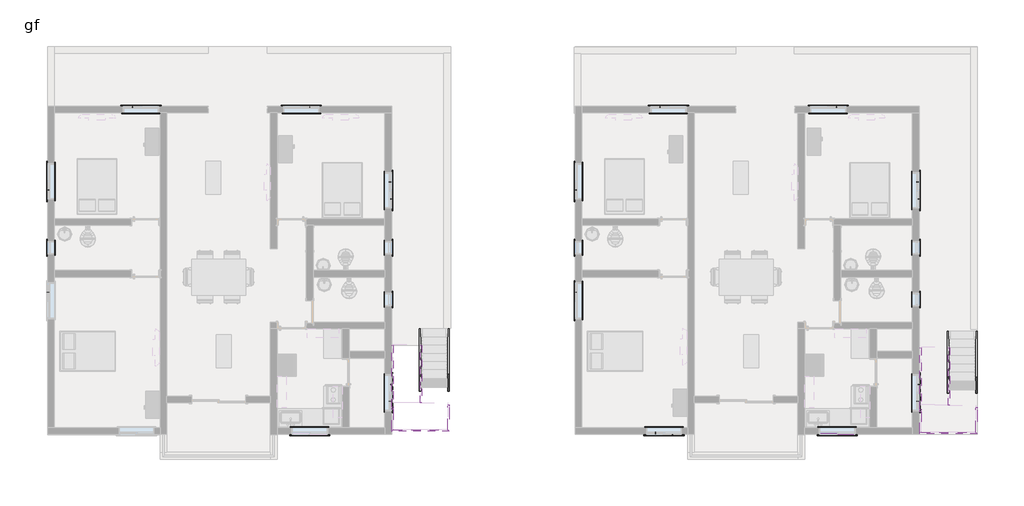
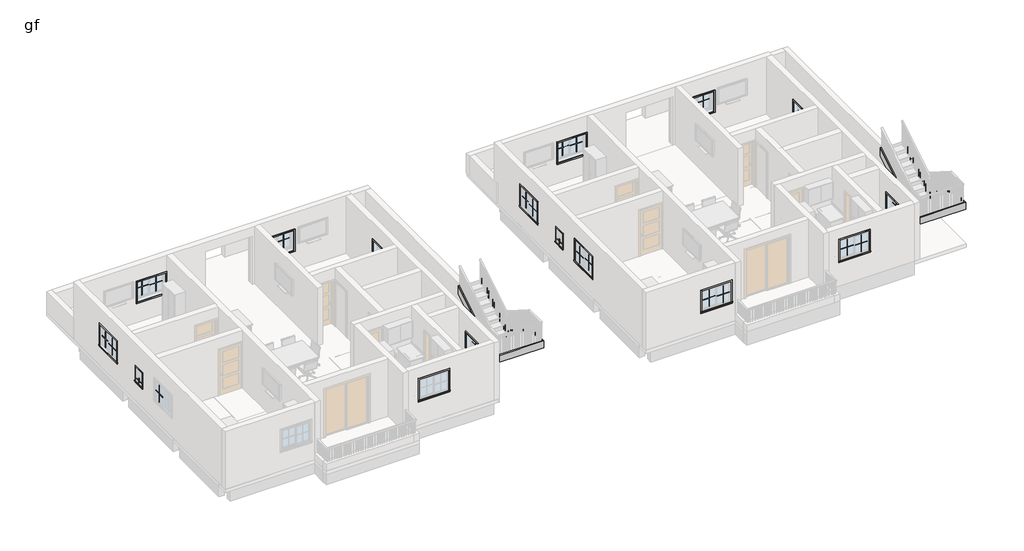
# One storey, part 8 of 8: 73 proxies, 14 members.
"""IFC4 building model written with IfcOpenShell, lengths in millimetres."""

from ifc_helpers import new_model, si_unit, frame, origin, place, context, project, spatial, polyline, outline, extrude, faceted_brep, transform, mapped, element, save
from components import muntin_pattern_2x2_muntin_pattern_2x2_0ac132d2, muntin_pattern_2x2_muntin_pattern_2x2_1fb5fae3, muntin_pattern_2x2_muntin_pattern_2x2_bb7dbb97, trim_window_exterior_flat_with_sill_c4e67c73, trim_window_exterior_flat_with_sill_729ce974, trim_window_exterior_flat_with_sill_e496db69, trim_window_interior_flat_picture_frame_cf1733af, trim_window_interior_flat_picture_frame_5593adf3, trim_window_interior_flat_picture_frame_58837336

model = new_model("IFC4")

# Units and contexts
model_context = context("Model", 3, world=origin())
ifc_project = project(units=[si_unit("LENGTHUNIT", "METRE", prefix="MILLI")], contexts=[model_context])

# Site, building, storey
site = spatial("IfcSite", under=ifc_project)
building = spatial("IfcBuilding", under=site)
storey = spatial("IfcBuildingStorey", under=building, Name="gf", Elevation=609.6)

# Proxies
placement = place(None, origin())
muntin_pattern_2x2_muntin_pattern_2x2_shape = muntin_pattern_2x2_muntin_pattern_2x2_0ac132d2(model_context)
element("IfcBuildingElementProxy", 1, Name="Muntin Pattern_2x2 : Muntin Pattern_2x2", ObjectType="Muntin Pattern_2x2 : Muntin Pattern_2x2", at=placement, inside=storey, context=model_context, shape_type="MappedRepresentation", body=[
    mapped(muntin_pattern_2x2_muntin_pattern_2x2_shape, transform((-12854.1368763, 6465.9185985, 1606.55), x_axis=(1.0, 0.0, 0.0), y_axis=(0.0, 1.0, 0.0), z_axis=(0.0, 0.0, 1.0))),
])
element("IfcBuildingElementProxy", 2, Name="Muntin Pattern_2x2 : Muntin Pattern_2x2", ObjectType="Muntin Pattern_2x2 : Muntin Pattern_2x2", at=placement, inside=storey, context=model_context, shape_type="MappedRepresentation", body=[
    mapped(muntin_pattern_2x2_muntin_pattern_2x2_shape, transform((-13422.4618763, 6510.3685985, 1606.55), x_axis=(1.0, 0.0, 0.0), y_axis=(0.0, 1.0, 0.0), z_axis=(0.0, 0.0, 1.0))),
])
element("IfcBuildingElementProxy", 3, Name="Muntin Pattern_2x2 : Muntin Pattern_2x2", ObjectType="Muntin Pattern_2x2 : Muntin Pattern_2x2", at=placement, inside=storey, context=model_context, shape_type="MappedRepresentation", body=[
    mapped(muntin_pattern_2x2_muntin_pattern_2x2_shape, transform((-16246.6243763, 4251.3560985, 1606.55), x_axis=(0.0, 1.0, 0.0), y_axis=(-1.0, 0.0, 0.0), z_axis=(0.0, 0.0, 1.0))),
])
element("IfcBuildingElementProxy", 4, Name="Muntin Pattern_2x2 : Muntin Pattern_2x2", ObjectType="Muntin Pattern_2x2 : Muntin Pattern_2x2", at=placement, inside=storey, context=model_context, shape_type="MappedRepresentation", body=[
    mapped(muntin_pattern_2x2_muntin_pattern_2x2_shape, transform((-16291.0743763, 3683.0310985, 1606.55), x_axis=(0.0, 1.0, 0.0), y_axis=(-1.0, 0.0, 0.0), z_axis=(0.0, 0.0, 1.0))),
])
element("IfcBuildingElementProxy", 5, Name="Muntin Pattern_2x2 : Muntin Pattern_2x2", ObjectType="Muntin Pattern_2x2 : Muntin Pattern_2x2", at=placement, inside=storey, context=model_context, shape_type="MappedRepresentation", body=[
    mapped(muntin_pattern_2x2_muntin_pattern_2x2_shape, transform((-4695.9743763, -3479.7689015, 1606.55), x_axis=(0.0, -1.0, 0.0), y_axis=(1.0, 0.0, 0.0), z_axis=(0.0, 0.0, 1.0))),
])
element("IfcBuildingElementProxy", 6, Name="Muntin Pattern_2x2 : Muntin Pattern_2x2", ObjectType="Muntin Pattern_2x2 : Muntin Pattern_2x2", at=placement, inside=storey, context=model_context, shape_type="MappedRepresentation", body=[
    mapped(muntin_pattern_2x2_muntin_pattern_2x2_shape, transform((-4651.5243763, -2911.4439015, 1606.55), x_axis=(0.0, -1.0, 0.0), y_axis=(1.0, 0.0, 0.0), z_axis=(0.0, 0.0, 1.0))),
])
element("IfcBuildingElementProxy", 7, Name="Muntin Pattern_2x2 : Muntin Pattern_2x2", ObjectType="Muntin Pattern_2x2 : Muntin Pattern_2x2", at=placement, inside=storey, context=model_context, shape_type="MappedRepresentation", body=[
    mapped(muntin_pattern_2x2_muntin_pattern_2x2_shape, transform((10167.1136273, -4551.3314015, 1835.15), x_axis=(-1.0, 0.0, 0.0), y_axis=(0.0, -1.0, 0.0), z_axis=(0.0, 0.0, 1.0))),
])
element("IfcBuildingElementProxy", 8, Name="Muntin Pattern_2x2 : Muntin Pattern_2x2", ObjectType="Muntin Pattern_2x2 : Muntin Pattern_2x2", at=placement, inside=storey, context=model_context, shape_type="MappedRepresentation", body=[
    mapped(muntin_pattern_2x2_muntin_pattern_2x2_shape, transform((10735.4386273, -4595.7814015, 1835.15), x_axis=(-1.0, 0.0, 0.0), y_axis=(0.0, -1.0, 0.0), z_axis=(0.0, 0.0, 1.0))),
])
element("IfcBuildingElementProxy", 9, Name="Muntin Pattern_2x2 : Muntin Pattern_2x2", ObjectType="Muntin Pattern_2x2 : Muntin Pattern_2x2", at=placement, inside=storey, context=model_context, shape_type="MappedRepresentation", body=[
    mapped(muntin_pattern_2x2_muntin_pattern_2x2_shape, transform((5020.4386273, 6465.9185985, 1606.55), x_axis=(1.0, 0.0, 0.0), y_axis=(0.0, 1.0, 0.0), z_axis=(0.0, 0.0, 1.0))),
])
element("IfcBuildingElementProxy", 10, Name="Muntin Pattern_2x2 : Muntin Pattern_2x2", ObjectType="Muntin Pattern_2x2 : Muntin Pattern_2x2", at=placement, inside=storey, context=model_context, shape_type="MappedRepresentation", body=[
    mapped(muntin_pattern_2x2_muntin_pattern_2x2_shape, transform((4452.1136273, 6510.3685985, 1606.55), x_axis=(1.0, 0.0, 0.0), y_axis=(0.0, 1.0, 0.0), z_axis=(0.0, 0.0, 1.0))),
])
element("IfcBuildingElementProxy", 11, Name="Muntin Pattern_2x2 : Muntin Pattern_2x2", ObjectType="Muntin Pattern_2x2 : Muntin Pattern_2x2", at=placement, inside=storey, context=model_context, shape_type="MappedRepresentation", body=[
    mapped(muntin_pattern_2x2_muntin_pattern_2x2_shape, transform((1627.9511273, 4251.3560985, 1606.55), x_axis=(0.0, 1.0, 0.0), y_axis=(-1.0, 0.0, 0.0), z_axis=(0.0, 0.0, 1.0))),
])
element("IfcBuildingElementProxy", 12, Name="Muntin Pattern_2x2 : Muntin Pattern_2x2", ObjectType="Muntin Pattern_2x2 : Muntin Pattern_2x2", at=placement, inside=storey, context=model_context, shape_type="MappedRepresentation", body=[
    mapped(muntin_pattern_2x2_muntin_pattern_2x2_shape, transform((1583.5011273, 3683.0310985, 1606.55), x_axis=(0.0, 1.0, 0.0), y_axis=(-1.0, 0.0, 0.0), z_axis=(0.0, 0.0, 1.0))),
])
element("IfcBuildingElementProxy", 13, Name="Muntin Pattern_2x2 : Muntin Pattern_2x2", ObjectType="Muntin Pattern_2x2 : Muntin Pattern_2x2", at=placement, inside=storey, context=model_context, shape_type="MappedRepresentation", body=[
    mapped(muntin_pattern_2x2_muntin_pattern_2x2_shape, transform((4299.7136273, -4551.3314015, 1606.55), x_axis=(-1.0, 0.0, 0.0), y_axis=(0.0, -1.0, 0.0), z_axis=(0.0, 0.0, 1.0))),
])
element("IfcBuildingElementProxy", 14, Name="Muntin Pattern_2x2 : Muntin Pattern_2x2", ObjectType="Muntin Pattern_2x2 : Muntin Pattern_2x2", at=placement, inside=storey, context=model_context, shape_type="MappedRepresentation", body=[
    mapped(muntin_pattern_2x2_muntin_pattern_2x2_shape, transform((4868.0386273, -4595.7814015, 1606.55), x_axis=(-1.0, 0.0, 0.0), y_axis=(0.0, -1.0, 0.0), z_axis=(0.0, 0.0, 1.0))),
])
element("IfcBuildingElementProxy", 15, Name="Muntin Pattern_2x2 : Muntin Pattern_2x2", ObjectType="Muntin Pattern_2x2 : Muntin Pattern_2x2", at=placement, inside=storey, context=model_context, shape_type="MappedRepresentation", body=[
    mapped(muntin_pattern_2x2_muntin_pattern_2x2_shape, transform((13178.6011273, -3479.7689015, 1606.55), x_axis=(0.0, -1.0, 0.0), y_axis=(1.0, 0.0, 0.0), z_axis=(0.0, 0.0, 1.0))),
])
element("IfcBuildingElementProxy", 16, Name="Muntin Pattern_2x2 : Muntin Pattern_2x2", ObjectType="Muntin Pattern_2x2 : Muntin Pattern_2x2", at=placement, inside=storey, context=model_context, shape_type="MappedRepresentation", body=[
    mapped(muntin_pattern_2x2_muntin_pattern_2x2_shape, transform((13223.0511273, -2911.4439015, 1606.55), x_axis=(0.0, -1.0, 0.0), y_axis=(1.0, 0.0, 0.0), z_axis=(0.0, 0.0, 1.0))),
])
muntin_pattern_2x2_muntin_pattern_2x2_2_shape = muntin_pattern_2x2_muntin_pattern_2x2_1fb5fae3(model_context)
element("IfcBuildingElementProxy", 17, Name="Muntin Pattern_2x2 : Muntin Pattern_2x2", ObjectType="Muntin Pattern_2x2 : Muntin Pattern_2x2", at=placement, inside=storey, context=model_context, shape_type="MappedRepresentation", body=[
    mapped(muntin_pattern_2x2_muntin_pattern_2x2_2_shape, transform((-4695.9743763, 3946.5560985, 1606.55), x_axis=(0.0, 1.0, 0.0), y_axis=(-1.0, 0.0, 0.0), z_axis=(0.0, 0.0, 1.0))),
])
element("IfcBuildingElementProxy", 18, Name="Muntin Pattern_2x2 : Muntin Pattern_2x2", ObjectType="Muntin Pattern_2x2 : Muntin Pattern_2x2", at=placement, inside=storey, context=model_context, shape_type="MappedRepresentation", body=[
    mapped(muntin_pattern_2x2_muntin_pattern_2x2_2_shape, transform((-4651.5243763, 3378.2310985, 1606.55), x_axis=(0.0, 1.0, 0.0), y_axis=(-1.0, 0.0, 0.0), z_axis=(0.0, 0.0, 1.0))),
])
element("IfcBuildingElementProxy", 19, Name="Muntin Pattern_2x2 : Muntin Pattern_2x2", ObjectType="Muntin Pattern_2x2 : Muntin Pattern_2x2", at=placement, inside=storey, context=model_context, shape_type="MappedRepresentation", body=[
    mapped(muntin_pattern_2x2_muntin_pattern_2x2_2_shape, transform((-7986.8618763, 6465.9185985, 1606.55), x_axis=(-1.0, 0.0, 0.0), y_axis=(0.0, -1.0, 0.0), z_axis=(0.0, 0.0, 1.0))),
])
element("IfcBuildingElementProxy", 20, Name="Muntin Pattern_2x2 : Muntin Pattern_2x2", ObjectType="Muntin Pattern_2x2 : Muntin Pattern_2x2", at=placement, inside=storey, context=model_context, shape_type="MappedRepresentation", body=[
    mapped(muntin_pattern_2x2_muntin_pattern_2x2_2_shape, transform((-7418.5368763, 6510.3685985, 1606.55), x_axis=(-1.0, 0.0, 0.0), y_axis=(0.0, -1.0, 0.0), z_axis=(0.0, 0.0, 1.0))),
])
element("IfcBuildingElementProxy", 21, Name="Muntin Pattern_2x2 : Muntin Pattern_2x2", ObjectType="Muntin Pattern_2x2 : Muntin Pattern_2x2", at=placement, inside=storey, context=model_context, shape_type="MappedRepresentation", body=[
    mapped(muntin_pattern_2x2_muntin_pattern_2x2_2_shape, transform((-16291.0743763, 212.7560985, 1606.55), x_axis=(0.0, -1.0, 0.0), y_axis=(1.0, 0.0, 0.0), z_axis=(0.0, 0.0, 1.0))),
])
element("IfcBuildingElementProxy", 22, Name="Muntin Pattern_2x2 : Muntin Pattern_2x2", ObjectType="Muntin Pattern_2x2 : Muntin Pattern_2x2", at=placement, inside=storey, context=model_context, shape_type="MappedRepresentation", body=[
    mapped(muntin_pattern_2x2_muntin_pattern_2x2_2_shape, transform((13178.6011273, 3946.5560985, 1606.55), x_axis=(0.0, 1.0, 0.0), y_axis=(-1.0, 0.0, 0.0), z_axis=(0.0, 0.0, 1.0))),
])
element("IfcBuildingElementProxy", 23, Name="Muntin Pattern_2x2 : Muntin Pattern_2x2", ObjectType="Muntin Pattern_2x2 : Muntin Pattern_2x2", at=placement, inside=storey, context=model_context, shape_type="MappedRepresentation", body=[
    mapped(muntin_pattern_2x2_muntin_pattern_2x2_2_shape, transform((13223.0511273, 3378.2310985, 1606.55), x_axis=(0.0, 1.0, 0.0), y_axis=(-1.0, 0.0, 0.0), z_axis=(0.0, 0.0, 1.0))),
])
element("IfcBuildingElementProxy", 24, Name="Muntin Pattern_2x2 : Muntin Pattern_2x2", ObjectType="Muntin Pattern_2x2 : Muntin Pattern_2x2", at=placement, inside=storey, context=model_context, shape_type="MappedRepresentation", body=[
    mapped(muntin_pattern_2x2_muntin_pattern_2x2_2_shape, transform((9862.3136273, 6465.9185985, 1606.55), x_axis=(-1.0, 0.0, 0.0), y_axis=(0.0, -1.0, 0.0), z_axis=(0.0, 0.0, 1.0))),
])
element("IfcBuildingElementProxy", 25, Name="Muntin Pattern_2x2 : Muntin Pattern_2x2", ObjectType="Muntin Pattern_2x2 : Muntin Pattern_2x2", at=placement, inside=storey, context=model_context, shape_type="MappedRepresentation", body=[
    mapped(muntin_pattern_2x2_muntin_pattern_2x2_2_shape, transform((10430.6386273, 6510.3685985, 1606.55), x_axis=(-1.0, 0.0, 0.0), y_axis=(0.0, -1.0, 0.0), z_axis=(0.0, 0.0, 1.0))),
])
element("IfcBuildingElementProxy", 26, Name="Muntin Pattern_2x2 : Muntin Pattern_2x2", ObjectType="Muntin Pattern_2x2 : Muntin Pattern_2x2", at=placement, inside=storey, context=model_context, shape_type="MappedRepresentation", body=[
    mapped(muntin_pattern_2x2_muntin_pattern_2x2_2_shape, transform((1627.9511273, -355.5689015, 1606.55), x_axis=(0.0, -1.0, 0.0), y_axis=(1.0, 0.0, 0.0), z_axis=(0.0, 0.0, 1.0))),
])
element("IfcBuildingElementProxy", 27, Name="Muntin Pattern_2x2 : Muntin Pattern_2x2", ObjectType="Muntin Pattern_2x2 : Muntin Pattern_2x2", at=placement, inside=storey, context=model_context, shape_type="MappedRepresentation", body=[
    mapped(muntin_pattern_2x2_muntin_pattern_2x2_2_shape, transform((1583.5011273, 212.7560985, 1606.55), x_axis=(0.0, -1.0, 0.0), y_axis=(1.0, 0.0, 0.0), z_axis=(0.0, 0.0, 1.0))),
])
muntin_pattern_2x2_muntin_pattern_2x2_3_shape = muntin_pattern_2x2_muntin_pattern_2x2_bb7dbb97(model_context)
element("IfcBuildingElementProxy", 28, Name="Muntin Pattern_2x2 : Muntin Pattern_2x2", ObjectType="Muntin Pattern_2x2 : Muntin Pattern_2x2", at=placement, inside=storey, context=model_context, shape_type="MappedRepresentation", body=[
    mapped(muntin_pattern_2x2_muntin_pattern_2x2_3_shape, transform((-4651.5243763, -33.3064015, 1562.1), x_axis=(0.0, 1.0, 0.0), y_axis=(-1.0, 0.0, 0.0), z_axis=(0.0, 0.0, 1.0))),
])
element("IfcBuildingElementProxy", 29, Name="Muntin Pattern_2x2 : Muntin Pattern_2x2", ObjectType="Muntin Pattern_2x2 : Muntin Pattern_2x2", at=placement, inside=storey, context=model_context, shape_type="MappedRepresentation", body=[
    mapped(muntin_pattern_2x2_muntin_pattern_2x2_3_shape, transform((-4651.5243763, 1719.2935985, 1562.1), x_axis=(0.0, 1.0, 0.0), y_axis=(-1.0, 0.0, 0.0), z_axis=(0.0, 0.0, 1.0))),
])
element("IfcBuildingElementProxy", 30, Name="Muntin Pattern_2x2 : Muntin Pattern_2x2", ObjectType="Muntin Pattern_2x2 : Muntin Pattern_2x2", at=placement, inside=storey, context=model_context, shape_type="MappedRepresentation", body=[
    mapped(muntin_pattern_2x2_muntin_pattern_2x2_3_shape, transform((-16291.0743763, 1719.2935985, 1562.1), x_axis=(0.0, -1.0, 0.0), y_axis=(1.0, 0.0, 0.0), z_axis=(0.0, 0.0, 1.0))),
])
element("IfcBuildingElementProxy", 31, Name="Muntin Pattern_2x2 : Muntin Pattern_2x2", ObjectType="Muntin Pattern_2x2 : Muntin Pattern_2x2", at=placement, inside=storey, context=model_context, shape_type="MappedRepresentation", body=[
    mapped(muntin_pattern_2x2_muntin_pattern_2x2_3_shape, transform((13223.0511273, -33.3064015, 1562.1), x_axis=(0.0, 1.0, 0.0), y_axis=(-1.0, 0.0, 0.0), z_axis=(0.0, 0.0, 1.0))),
])
element("IfcBuildingElementProxy", 32, Name="Muntin Pattern_2x2 : Muntin Pattern_2x2", ObjectType="Muntin Pattern_2x2 : Muntin Pattern_2x2", at=placement, inside=storey, context=model_context, shape_type="MappedRepresentation", body=[
    mapped(muntin_pattern_2x2_muntin_pattern_2x2_3_shape, transform((13223.0511273, 1719.2935985, 1562.1), x_axis=(0.0, 1.0, 0.0), y_axis=(-1.0, 0.0, 0.0), z_axis=(0.0, 0.0, 1.0))),
])
element("IfcBuildingElementProxy", 33, Name="Muntin Pattern_2x2 : Muntin Pattern_2x2", ObjectType="Muntin Pattern_2x2 : Muntin Pattern_2x2", at=placement, inside=storey, context=model_context, shape_type="MappedRepresentation", body=[
    mapped(muntin_pattern_2x2_muntin_pattern_2x2_3_shape, transform((1583.5011273, 1719.2935985, 1562.1), x_axis=(0.0, -1.0, 0.0), y_axis=(1.0, 0.0, 0.0), z_axis=(0.0, 0.0, 1.0))),
])
trim_window_exterior_flat_with_sill_shape = trim_window_exterior_flat_with_sill_c4e67c73(model_context)
element("IfcBuildingElementProxy", 34, Name="Trim-Window-Exterior-Flat : with Sill", ObjectType="Trim-Window-Exterior-Flat : with Sill", at=placement, inside=storey, context=model_context, shape_type="MappedRepresentation", body=[
    mapped(trim_window_exterior_flat_with_sill_shape, transform((-7423.2993763, -4605.3064015, 2667.0), x_axis=(1.0, 0.0, 0.0), y_axis=(0.0, 0.0, 1.0), z_axis=(0.0, -1.0, 0.0))),
])
element("IfcBuildingElementProxy", 35, Name="Trim-Window-Exterior-Flat : with Sill", ObjectType="Trim-Window-Exterior-Flat : with Sill", at=placement, inside=storey, context=model_context, shape_type="MappedRepresentation", body=[
    mapped(trim_window_exterior_flat_with_sill_shape, transform((-13138.2993763, 6519.8935985, 2438.4), x_axis=(-1.0, 0.0, 0.0), y_axis=(0.0, 0.0, 1.0), z_axis=(0.0, 1.0, 0.0))),
])
element("IfcBuildingElementProxy", 36, Name="Trim-Window-Exterior-Flat : with Sill", ObjectType="Trim-Window-Exterior-Flat : with Sill", at=placement, inside=storey, context=model_context, shape_type="MappedRepresentation", body=[
    mapped(trim_window_exterior_flat_with_sill_shape, transform((-16300.5993763, 3967.1935985, 2438.4), x_axis=(0.0, -1.0, 0.0), y_axis=(0.0, 0.0, 1.0), z_axis=(-1.0, 0.0, 0.0))),
])
element("IfcBuildingElementProxy", 37, Name="Trim-Window-Exterior-Flat : with Sill", ObjectType="Trim-Window-Exterior-Flat : with Sill", at=placement, inside=storey, context=model_context, shape_type="MappedRepresentation", body=[
    mapped(trim_window_exterior_flat_with_sill_shape, transform((-4641.9993763, -3195.6064015, 2438.4), x_axis=(0.0, 1.0, 0.0), y_axis=(0.0, 0.0, 1.0), z_axis=(1.0, 0.0, 0.0))),
])
element("IfcBuildingElementProxy", 38, Name="Trim-Window-Exterior-Flat : with Sill", ObjectType="Trim-Window-Exterior-Flat : with Sill", at=placement, inside=storey, context=model_context, shape_type="MappedRepresentation", body=[
    mapped(trim_window_exterior_flat_with_sill_shape, transform((10451.2761273, -4605.3064015, 2667.0), x_axis=(1.0, 0.0, 0.0), y_axis=(0.0, 0.0, 1.0), z_axis=(0.0, -1.0, 0.0))),
])
element("IfcBuildingElementProxy", 39, Name="Trim-Window-Exterior-Flat : with Sill", ObjectType="Trim-Window-Exterior-Flat : with Sill", at=placement, inside=storey, context=model_context, shape_type="MappedRepresentation", body=[
    mapped(trim_window_exterior_flat_with_sill_shape, transform((4736.2761273, 6519.8935985, 2438.4), x_axis=(-1.0, 0.0, 0.0), y_axis=(0.0, 0.0, 1.0), z_axis=(0.0, 1.0, 0.0))),
])
element("IfcBuildingElementProxy", 40, Name="Trim-Window-Exterior-Flat : with Sill", ObjectType="Trim-Window-Exterior-Flat : with Sill", at=placement, inside=storey, context=model_context, shape_type="MappedRepresentation", body=[
    mapped(trim_window_exterior_flat_with_sill_shape, transform((1573.9761273, 3967.1935985, 2438.4), x_axis=(0.0, -1.0, 0.0), y_axis=(0.0, 0.0, 1.0), z_axis=(-1.0, 0.0, 0.0))),
])
element("IfcBuildingElementProxy", 41, Name="Trim-Window-Exterior-Flat : with Sill", ObjectType="Trim-Window-Exterior-Flat : with Sill", at=placement, inside=storey, context=model_context, shape_type="MappedRepresentation", body=[
    mapped(trim_window_exterior_flat_with_sill_shape, transform((4583.8761273, -4605.3064015, 2438.4), x_axis=(1.0, 0.0, 0.0), y_axis=(0.0, 0.0, 1.0), z_axis=(0.0, -1.0, 0.0))),
])
element("IfcBuildingElementProxy", 42, Name="Trim-Window-Exterior-Flat : with Sill", ObjectType="Trim-Window-Exterior-Flat : with Sill", at=placement, inside=storey, context=model_context, shape_type="MappedRepresentation", body=[
    mapped(trim_window_exterior_flat_with_sill_shape, transform((13232.5761273, -3195.6064015, 2438.4), x_axis=(0.0, 1.0, 0.0), y_axis=(0.0, 0.0, 1.0), z_axis=(1.0, 0.0, 0.0))),
])
trim_window_exterior_flat_with_sill_2_shape = trim_window_exterior_flat_with_sill_729ce974(model_context)
element("IfcBuildingElementProxy", 43, Name="Trim-Window-Exterior-Flat : with Sill", ObjectType="Trim-Window-Exterior-Flat : with Sill", at=placement, inside=storey, context=model_context, shape_type="MappedRepresentation", body=[
    mapped(trim_window_exterior_flat_with_sill_2_shape, transform((-4641.9993763, 3662.3935985, 2438.4), x_axis=(0.0, -1.0, 0.0), y_axis=(0.0, 0.0, -1.0), z_axis=(1.0, 0.0, 0.0))),
])
element("IfcBuildingElementProxy", 44, Name="Trim-Window-Exterior-Flat : with Sill", ObjectType="Trim-Window-Exterior-Flat : with Sill", at=placement, inside=storey, context=model_context, shape_type="MappedRepresentation", body=[
    mapped(trim_window_exterior_flat_with_sill_2_shape, transform((-7702.6993763, 6519.8935985, 2438.4), x_axis=(1.0, 0.0, 0.0), y_axis=(0.0, 0.0, -1.0), z_axis=(0.0, 1.0, 0.0))),
])
element("IfcBuildingElementProxy", 45, Name="Trim-Window-Exterior-Flat : with Sill", ObjectType="Trim-Window-Exterior-Flat : with Sill", at=placement, inside=storey, context=model_context, shape_type="MappedRepresentation", body=[
    mapped(trim_window_exterior_flat_with_sill_2_shape, transform((13232.5761273, 3662.3935985, 2438.4), x_axis=(0.0, -1.0, 0.0), y_axis=(0.0, 0.0, -1.0), z_axis=(1.0, 0.0, 0.0))),
])
element("IfcBuildingElementProxy", 46, Name="Trim-Window-Exterior-Flat : with Sill", ObjectType="Trim-Window-Exterior-Flat : with Sill", at=placement, inside=storey, context=model_context, shape_type="MappedRepresentation", body=[
    mapped(trim_window_exterior_flat_with_sill_2_shape, transform((10146.4761273, 6519.8935985, 2438.4), x_axis=(1.0, 0.0, 0.0), y_axis=(0.0, 0.0, -1.0), z_axis=(0.0, 1.0, 0.0))),
])
element("IfcBuildingElementProxy", 47, Name="Trim-Window-Exterior-Flat : with Sill", ObjectType="Trim-Window-Exterior-Flat : with Sill", at=placement, inside=storey, context=model_context, shape_type="MappedRepresentation", body=[
    mapped(trim_window_exterior_flat_with_sill_2_shape, transform((1573.9761273, -71.4064015, 2438.4), x_axis=(0.0, 1.0, 0.0), y_axis=(0.0, 0.0, -1.0), z_axis=(-1.0, 0.0, 0.0))),
])
trim_window_exterior_flat_with_sill_3_shape = trim_window_exterior_flat_with_sill_e496db69(model_context)
element("IfcBuildingElementProxy", 48, Name="Trim-Window-Exterior-Flat : with Sill", ObjectType="Trim-Window-Exterior-Flat : with Sill", at=placement, inside=storey, context=model_context, shape_type="MappedRepresentation", body=[
    mapped(trim_window_exterior_flat_with_sill_3_shape, transform((-4641.9993763, -33.3064015, 2133.6), x_axis=(0.0, 1.0, 0.0), y_axis=(0.0, 0.0, 1.0), z_axis=(1.0, 0.0, 0.0))),
])
element("IfcBuildingElementProxy", 49, Name="Trim-Window-Exterior-Flat : with Sill", ObjectType="Trim-Window-Exterior-Flat : with Sill", at=placement, inside=storey, context=model_context, shape_type="MappedRepresentation", body=[
    mapped(trim_window_exterior_flat_with_sill_3_shape, transform((-4641.9993763, 1719.2935985, 2133.6), x_axis=(0.0, 1.0, 0.0), y_axis=(0.0, 0.0, 1.0), z_axis=(1.0, 0.0, 0.0))),
])
element("IfcBuildingElementProxy", 50, Name="Trim-Window-Exterior-Flat : with Sill", ObjectType="Trim-Window-Exterior-Flat : with Sill", at=placement, inside=storey, context=model_context, shape_type="MappedRepresentation", body=[
    mapped(trim_window_exterior_flat_with_sill_3_shape, transform((-16300.5993763, 1719.2935985, 2133.6), x_axis=(0.0, -1.0, 0.0), y_axis=(0.0, 0.0, 1.0), z_axis=(-1.0, 0.0, 0.0))),
])
element("IfcBuildingElementProxy", 51, Name="Trim-Window-Exterior-Flat : with Sill", ObjectType="Trim-Window-Exterior-Flat : with Sill", at=placement, inside=storey, context=model_context, shape_type="MappedRepresentation", body=[
    mapped(trim_window_exterior_flat_with_sill_3_shape, transform((13232.5761273, -33.3064015, 2133.6), x_axis=(0.0, 1.0, 0.0), y_axis=(0.0, 0.0, 1.0), z_axis=(1.0, 0.0, 0.0))),
])
element("IfcBuildingElementProxy", 52, Name="Trim-Window-Exterior-Flat : with Sill", ObjectType="Trim-Window-Exterior-Flat : with Sill", at=placement, inside=storey, context=model_context, shape_type="MappedRepresentation", body=[
    mapped(trim_window_exterior_flat_with_sill_3_shape, transform((13232.5761273, 1719.2935985, 2133.6), x_axis=(0.0, 1.0, 0.0), y_axis=(0.0, 0.0, 1.0), z_axis=(1.0, 0.0, 0.0))),
])
element("IfcBuildingElementProxy", 53, Name="Trim-Window-Exterior-Flat : with Sill", ObjectType="Trim-Window-Exterior-Flat : with Sill", at=placement, inside=storey, context=model_context, shape_type="MappedRepresentation", body=[
    mapped(trim_window_exterior_flat_with_sill_3_shape, transform((1573.9761273, 1719.2935985, 2133.6), x_axis=(0.0, -1.0, 0.0), y_axis=(0.0, 0.0, 1.0), z_axis=(-1.0, 0.0, 0.0))),
])
trim_window_interior_flat_picture_frame_shape = trim_window_interior_flat_picture_frame_cf1733af(model_context)
element("IfcBuildingElementProxy", 54, Name="Trim-Window-Interior-Flat : Picture Frame", ObjectType="Trim-Window-Interior-Flat : Picture Frame", at=placement, inside=storey, context=model_context, shape_type="MappedRepresentation", body=[
    mapped(trim_window_interior_flat_picture_frame_shape, transform((-7423.2993763, -4376.7064015, 2667.0), x_axis=(-1.0, 0.0, 0.0), y_axis=(0.0, 0.0, 1.0), z_axis=(0.0, 1.0, 0.0))),
])
element("IfcBuildingElementProxy", 55, Name="Trim-Window-Interior-Flat : Picture Frame", ObjectType="Trim-Window-Interior-Flat : Picture Frame", at=placement, inside=storey, context=model_context, shape_type="MappedRepresentation", body=[
    mapped(trim_window_interior_flat_picture_frame_shape, transform((-13138.2993763, 6291.2935985, 2438.4), x_axis=(1.0, 0.0, 0.0), y_axis=(0.0, 0.0, 1.0), z_axis=(0.0, -1.0, 0.0))),
])
element("IfcBuildingElementProxy", 56, Name="Trim-Window-Interior-Flat : Picture Frame", ObjectType="Trim-Window-Interior-Flat : Picture Frame", at=placement, inside=storey, context=model_context, shape_type="MappedRepresentation", body=[
    mapped(trim_window_interior_flat_picture_frame_shape, transform((-16071.9993763, 3967.1935985, 2438.4), x_axis=(0.0, 1.0, 0.0), y_axis=(0.0, 0.0, 1.0), z_axis=(1.0, 0.0, 0.0))),
])
element("IfcBuildingElementProxy", 57, Name="Trim-Window-Interior-Flat : Picture Frame", ObjectType="Trim-Window-Interior-Flat : Picture Frame", at=placement, inside=storey, context=model_context, shape_type="MappedRepresentation", body=[
    mapped(trim_window_interior_flat_picture_frame_shape, transform((-4870.5993763, -3195.6064015, 2438.4), x_axis=(0.0, -1.0, 0.0), y_axis=(0.0, 0.0, 1.0), z_axis=(-1.0, 0.0, 0.0))),
])
element("IfcBuildingElementProxy", 58, Name="Trim-Window-Interior-Flat : Picture Frame", ObjectType="Trim-Window-Interior-Flat : Picture Frame", at=placement, inside=storey, context=model_context, shape_type="MappedRepresentation", body=[
    mapped(trim_window_interior_flat_picture_frame_shape, transform((10451.2761273, -4376.7064015, 2667.0), x_axis=(-1.0, 0.0, 0.0), y_axis=(0.0, 0.0, 1.0), z_axis=(0.0, 1.0, 0.0))),
])
element("IfcBuildingElementProxy", 59, Name="Trim-Window-Interior-Flat : Picture Frame", ObjectType="Trim-Window-Interior-Flat : Picture Frame", at=placement, inside=storey, context=model_context, shape_type="MappedRepresentation", body=[
    mapped(trim_window_interior_flat_picture_frame_shape, transform((4736.2761273, 6291.2935985, 2438.4), x_axis=(1.0, 0.0, 0.0), y_axis=(0.0, 0.0, 1.0), z_axis=(0.0, -1.0, 0.0))),
])
element("IfcBuildingElementProxy", 60, Name="Trim-Window-Interior-Flat : Picture Frame", ObjectType="Trim-Window-Interior-Flat : Picture Frame", at=placement, inside=storey, context=model_context, shape_type="MappedRepresentation", body=[
    mapped(trim_window_interior_flat_picture_frame_shape, transform((1802.5761273, 3967.1935985, 2438.4), x_axis=(0.0, 1.0, 0.0), y_axis=(0.0, 0.0, 1.0), z_axis=(1.0, 0.0, 0.0))),
])
element("IfcBuildingElementProxy", 61, Name="Trim-Window-Interior-Flat : Picture Frame", ObjectType="Trim-Window-Interior-Flat : Picture Frame", at=placement, inside=storey, context=model_context, shape_type="MappedRepresentation", body=[
    mapped(trim_window_interior_flat_picture_frame_shape, transform((4583.8761273, -4376.7064015, 2438.4), x_axis=(-1.0, 0.0, 0.0), y_axis=(0.0, 0.0, 1.0), z_axis=(0.0, 1.0, 0.0))),
])
element("IfcBuildingElementProxy", 62, Name="Trim-Window-Interior-Flat : Picture Frame", ObjectType="Trim-Window-Interior-Flat : Picture Frame", at=placement, inside=storey, context=model_context, shape_type="MappedRepresentation", body=[
    mapped(trim_window_interior_flat_picture_frame_shape, transform((13003.9761273, -3195.6064015, 2438.4), x_axis=(0.0, -1.0, 0.0), y_axis=(0.0, 0.0, 1.0), z_axis=(-1.0, 0.0, 0.0))),
])
trim_window_interior_flat_picture_frame_2_shape = trim_window_interior_flat_picture_frame_5593adf3(model_context)
element("IfcBuildingElementProxy", 63, Name="Trim-Window-Interior-Flat : Picture Frame", ObjectType="Trim-Window-Interior-Flat : Picture Frame", at=placement, inside=storey, context=model_context, shape_type="MappedRepresentation", body=[
    mapped(trim_window_interior_flat_picture_frame_2_shape, transform((-4870.5993763, 3662.3935985, 2438.4), x_axis=(0.0, 1.0, 0.0), y_axis=(0.0, 0.0, -1.0), z_axis=(-1.0, 0.0, 0.0))),
])
element("IfcBuildingElementProxy", 64, Name="Trim-Window-Interior-Flat : Picture Frame", ObjectType="Trim-Window-Interior-Flat : Picture Frame", at=placement, inside=storey, context=model_context, shape_type="MappedRepresentation", body=[
    mapped(trim_window_interior_flat_picture_frame_2_shape, transform((-7702.6993763, 6291.2935985, 2438.4), x_axis=(-1.0, 0.0, 0.0), y_axis=(0.0, 0.0, -1.0), z_axis=(0.0, -1.0, 0.0))),
])
element("IfcBuildingElementProxy", 65, Name="Trim-Window-Interior-Flat : Picture Frame", ObjectType="Trim-Window-Interior-Flat : Picture Frame", at=placement, inside=storey, context=model_context, shape_type="MappedRepresentation", body=[
    mapped(trim_window_interior_flat_picture_frame_2_shape, transform((13003.9761273, 3662.3935985, 2438.4), x_axis=(0.0, 1.0, 0.0), y_axis=(0.0, 0.0, -1.0), z_axis=(-1.0, 0.0, 0.0))),
])
element("IfcBuildingElementProxy", 66, Name="Trim-Window-Interior-Flat : Picture Frame", ObjectType="Trim-Window-Interior-Flat : Picture Frame", at=placement, inside=storey, context=model_context, shape_type="MappedRepresentation", body=[
    mapped(trim_window_interior_flat_picture_frame_2_shape, transform((10146.4761273, 6291.2935985, 2438.4), x_axis=(-1.0, 0.0, 0.0), y_axis=(0.0, 0.0, -1.0), z_axis=(0.0, -1.0, 0.0))),
])
element("IfcBuildingElementProxy", 67, Name="Trim-Window-Interior-Flat : Picture Frame", ObjectType="Trim-Window-Interior-Flat : Picture Frame", at=placement, inside=storey, context=model_context, shape_type="MappedRepresentation", body=[
    mapped(trim_window_interior_flat_picture_frame_2_shape, transform((1802.5761273, -71.4064015, 2438.4), x_axis=(0.0, -1.0, 0.0), y_axis=(0.0, 0.0, -1.0), z_axis=(1.0, 0.0, 0.0))),
])
trim_window_interior_flat_picture_frame_3_shape = trim_window_interior_flat_picture_frame_58837336(model_context)
element("IfcBuildingElementProxy", 68, Name="Trim-Window-Interior-Flat : Picture Frame", ObjectType="Trim-Window-Interior-Flat : Picture Frame", at=placement, inside=storey, context=model_context, shape_type="MappedRepresentation", body=[
    mapped(trim_window_interior_flat_picture_frame_3_shape, transform((-4870.5993763, -33.3064015, 2133.6), x_axis=(0.0, -1.0, 0.0), y_axis=(0.0, 0.0, 1.0), z_axis=(-1.0, 0.0, 0.0))),
])
element("IfcBuildingElementProxy", 69, Name="Trim-Window-Interior-Flat : Picture Frame", ObjectType="Trim-Window-Interior-Flat : Picture Frame", at=placement, inside=storey, context=model_context, shape_type="MappedRepresentation", body=[
    mapped(trim_window_interior_flat_picture_frame_3_shape, transform((-4870.5993763, 1719.2935985, 2133.6), x_axis=(0.0, -1.0, 0.0), y_axis=(0.0, 0.0, 1.0), z_axis=(-1.0, 0.0, 0.0))),
])
element("IfcBuildingElementProxy", 70, Name="Trim-Window-Interior-Flat : Picture Frame", ObjectType="Trim-Window-Interior-Flat : Picture Frame", at=placement, inside=storey, context=model_context, shape_type="MappedRepresentation", body=[
    mapped(trim_window_interior_flat_picture_frame_3_shape, transform((-16071.9993763, 1719.2935985, 2133.6), x_axis=(0.0, 1.0, 0.0), y_axis=(0.0, 0.0, 1.0), z_axis=(1.0, 0.0, 0.0))),
])
element("IfcBuildingElementProxy", 71, Name="Trim-Window-Interior-Flat : Picture Frame", ObjectType="Trim-Window-Interior-Flat : Picture Frame", at=placement, inside=storey, context=model_context, shape_type="MappedRepresentation", body=[
    mapped(trim_window_interior_flat_picture_frame_3_shape, transform((13003.9761273, -33.3064015, 2133.6), x_axis=(0.0, -1.0, 0.0), y_axis=(0.0, 0.0, 1.0), z_axis=(-1.0, 0.0, 0.0))),
])
element("IfcBuildingElementProxy", 72, Name="Trim-Window-Interior-Flat : Picture Frame", ObjectType="Trim-Window-Interior-Flat : Picture Frame", at=placement, inside=storey, context=model_context, shape_type="MappedRepresentation", body=[
    mapped(trim_window_interior_flat_picture_frame_3_shape, transform((13003.9761273, 1719.2935985, 2133.6), x_axis=(0.0, -1.0, 0.0), y_axis=(0.0, 0.0, 1.0), z_axis=(-1.0, 0.0, 0.0))),
])
element("IfcBuildingElementProxy", 73, Name="Trim-Window-Interior-Flat : Picture Frame", ObjectType="Trim-Window-Interior-Flat : Picture Frame", at=placement, inside=storey, context=model_context, shape_type="MappedRepresentation", body=[
    mapped(trim_window_interior_flat_picture_frame_3_shape, transform((1802.5761273, 1719.2935985, 2133.6), x_axis=(0.0, 1.0, 0.0), y_axis=(0.0, 0.0, 1.0), z_axis=(1.0, 0.0, 0.0))),
])

# Members
element("IfcMember", 74, ObjectType="Stringer - 2\" Width", at=placement, inside=storey, context=model_context, shape_type="SweptSolid", body=[
    extrude(outline(polyline([(-1023.9064015, 824.6106437), (-1023.9064015, 609.6), (-1253.7619309, 609.6), (-3688.5333594, 2159.0), (-3599.77539, 2463.8), (-1023.9064015, 824.6106437)])), frame((-2736.9993763, 0.0, 0.0), z_axis=(1.0, 0.0, 0.0), x_axis=(0.0, 1.0, 0.0)), (0.0, 0.0, 1.0), 50.8),
])
element("IfcMember", 75, ObjectType="Stringer - 2\" Width", at=placement, inside=storey, context=model_context, shape_type="SweptSolid", body=[
    extrude(outline(polyline([(-1023.9064015, 824.6106437), (-1023.9064015, 609.6), (-1253.7619309, 609.6), (-3487.7064015, 2031.2010268), (-3487.7064015, 2392.483371), (-1023.9064015, 824.6106437)])), frame((-3702.1993763, 0.0, 0.0), z_axis=(1.0, 0.0, 0.0), x_axis=(0.0, 1.0, 0.0)), (0.0, 0.0, 1.0), 50.8),
])
element("IfcMember", 76, ObjectType="Stringer - 2\" Width", at=placement, inside=storey, context=model_context, shape_type="SweptSolid", body=[
    extrude(outline(polyline([(-3667.8794436, 2159.0), (-3756.637413, 2463.8), (-1582.7064015, 3847.2106437), (-1582.7064015, 3485.9282995), (-3667.8794436, 2159.0)])), frame((-4641.9993763, 0.0, 0.0), z_axis=(1.0, 0.0, 0.0), x_axis=(0.0, 1.0, 0.0)), (0.0, 0.0, 1.0), 50.8),
])
element("IfcMember", 77, ObjectType="Stringer - 2\" Width", at=placement, inside=storey, context=model_context, shape_type="SweptSolid", body=[
    extrude(outline(polyline([(-3538.5064015, 2241.3282995), (-3538.5064015, 2602.6106437), (-1582.7064015, 3847.2106437), (-1582.7064015, 3485.9282995), (-3538.5064015, 2241.3282995)])), frame((-3676.7993763, 0.0, 0.0), z_axis=(1.0, 0.0, 0.0), x_axis=(0.0, 1.0, 0.0)), (0.0, 0.0, 1.0), 50.8),
])
element("IfcMember", 78, ObjectType="Stringer - 2\" Width", at=placement, inside=storey, context=model_context, shape_type="Brep", body=[
    faceted_brep([(-4591.1993763, -3756.637413, 2463.8), (-4641.9993763, -3756.637413, 2463.8), (-4641.9993763, -4503.7064015, 2463.8), (-4591.1993763, -4452.9064015, 2463.8), (-4591.1993763, -3667.8794436, 2159.0), (-4591.1993763, -4452.9064015, 2159.0), (-4641.9993763, -3667.8794436, 2159.0), (-4641.9993763, -4503.7064015, 2159.0)], [[[0, 1, 2, 3]], [[4, 0, 3, 5]], [[6, 4, 5, 7]], [[1, 6, 7, 2]], [[1, 0, 4, 6]], [[2, 7, 5, 3]]]),
])
element("IfcMember", 79, ObjectType="Stringer - 2\" Width", at=placement, inside=storey, context=model_context, shape_type="SweptSolid", body=[
    extrude(outline(polyline([(-4641.9993763, -4503.7064015), (-4591.1993763, -4452.9064015), (-2736.9993763, -4452.9064015), (-2686.1993763, -4503.7064015), (-4641.9993763, -4503.7064015)])), frame((0.0, 0.0, 2159.0), z_axis=(0.0, 0.0, 1.0), x_axis=(1.0, 0.0, 0.0)), (0.0, 0.0, 1.0), 304.8),
])
element("IfcMember", 80, ObjectType="Stringer - 2\" Width", at=placement, inside=storey, context=model_context, shape_type="Brep", body=[
    faceted_brep([(-2736.9993763, -4452.9064015, 2463.8), (-2686.1993763, -4503.7064015, 2463.8), (-2686.1993763, -3599.77539, 2463.8), (-2736.9993763, -3599.77539, 2463.8), (-2736.9993763, -4452.9064015, 2159.0), (-2736.9993763, -3688.5333594, 2159.0), (-2686.1993763, -4503.7064015, 2159.0), (-2686.1993763, -3688.5333594, 2159.0)], [[[0, 1, 2, 3]], [[4, 0, 3, 5]], [[6, 4, 5, 7]], [[1, 6, 7, 2]], [[1, 0, 4, 6]], [[2, 7, 5, 3]]]),
])
element("IfcMember", 81, ObjectType="Stringer - 2\" Width", at=placement, inside=storey, context=model_context, shape_type="SweptSolid", body=[
    extrude(outline(polyline([(-1100.1064015, 824.6106437), (-1100.1064015, 609.6), (-1329.9619309, 609.6), (-3764.7333594, 2159.0), (-3675.97539, 2463.8), (-1100.1064015, 824.6106437)])), frame((15150.2761273, 0.0, 0.0), z_axis=(1.0, 0.0, 0.0), x_axis=(0.0, 1.0, 0.0)), (0.0, 0.0, 1.0), 50.8),
])
element("IfcMember", 82, ObjectType="Stringer - 2\" Width", at=placement, inside=storey, context=model_context, shape_type="SweptSolid", body=[
    extrude(outline(polyline([(-1100.1064015, 824.6106437), (-1100.1064015, 609.6), (-1329.9619309, 609.6), (-3563.9064015, 2031.2010268), (-3563.9064015, 2392.483371), (-1100.1064015, 824.6106437)])), frame((14185.0761273, 0.0, 0.0), z_axis=(1.0, 0.0, 0.0), x_axis=(0.0, 1.0, 0.0)), (0.0, 0.0, 1.0), 50.8),
])
element("IfcMember", 83, ObjectType="Stringer - 2\" Width", at=placement, inside=storey, context=model_context, shape_type="SweptSolid", body=[
    extrude(outline(polyline([(-3744.0794436, 2159.0), (-3832.837413, 2463.8), (-1658.9064015, 3847.2106437), (-1658.9064015, 3485.9282995), (-3744.0794436, 2159.0)])), frame((13245.2761273, 0.0, 0.0), z_axis=(1.0, 0.0, 0.0), x_axis=(0.0, 1.0, 0.0)), (0.0, 0.0, 1.0), 50.8),
])
element("IfcMember", 84, ObjectType="Stringer - 2\" Width", at=placement, inside=storey, context=model_context, shape_type="SweptSolid", body=[
    extrude(outline(polyline([(-3614.7064015, 2241.3282995), (-3614.7064015, 2602.6106437), (-1658.9064015, 3847.2106437), (-1658.9064015, 3485.9282995), (-3614.7064015, 2241.3282995)])), frame((14210.4761273, 0.0, 0.0), z_axis=(1.0, 0.0, 0.0), x_axis=(0.0, 1.0, 0.0)), (0.0, 0.0, 1.0), 50.8),
])
element("IfcMember", 85, ObjectType="Stringer - 2\" Width", at=placement, inside=storey, context=model_context, shape_type="Brep", body=[
    faceted_brep([(13296.0761273, -3832.837413, 2463.8), (13245.2761273, -3832.837413, 2463.8), (13245.2761273, -4579.9064015, 2463.8), (13296.0761273, -4529.1064015, 2463.8), (13296.0761273, -3744.0794436, 2159.0), (13296.0761273, -4529.1064015, 2159.0), (13245.2761273, -3744.0794436, 2159.0), (13245.2761273, -4579.9064015, 2159.0)], [[[0, 1, 2, 3]], [[4, 0, 3, 5]], [[6, 4, 5, 7]], [[1, 6, 7, 2]], [[1, 0, 4, 6]], [[2, 7, 5, 3]]]),
])
element("IfcMember", 86, ObjectType="Stringer - 2\" Width", at=placement, inside=storey, context=model_context, shape_type="SweptSolid", body=[
    extrude(outline(polyline([(13245.2761273, -4579.9064015), (13296.0761273, -4529.1064015), (15150.2761273, -4529.1064015), (15201.0761273, -4579.9064015), (13245.2761273, -4579.9064015)])), frame((0.0, 0.0, 2159.0), z_axis=(0.0, 0.0, 1.0), x_axis=(1.0, 0.0, 0.0)), (0.0, 0.0, 1.0), 304.8),
])
element("IfcMember", 87, ObjectType="Stringer - 2\" Width", at=placement, inside=storey, context=model_context, shape_type="Brep", body=[
    faceted_brep([(15150.2761273, -4529.1064015, 2463.8), (15201.0761273, -4579.9064015, 2463.8), (15201.0761273, -3675.97539, 2463.8), (15150.2761273, -3675.97539, 2463.8), (15150.2761273, -4529.1064015, 2159.0), (15150.2761273, -3764.7333594, 2159.0), (15201.0761273, -4579.9064015, 2159.0), (15201.0761273, -3764.7333594, 2159.0)], [[[0, 1, 2, 3]], [[4, 0, 3, 5]], [[6, 4, 5, 7]], [[1, 6, 7, 2]], [[1, 0, 4, 6]], [[2, 7, 5, 3]]]),
])

save(model, "model.ifc")

# Revit data of these elements
# Type "Muntin Pattern_2x2 : Muntin Pattern_2x2"
#   Width [instance default] = 4' - 0"
#   Thickness = 0' - 0 1/2"
#   Height [instance default] = 4' - 0"
#   Distance = 0' - 0 3/4"
#   Interior Material [instance default] = none
#   Exterior Material [instance default] = none
#   Default Elevation = 0
# Type "Trim-Window-Exterior-Flat : with Sill"
#   Trim Width = 0' - 2 1/4"
#   Trim Thickness_Picture Frame = 0' - 1 1/4"
#   Trim Thickness_with Sill = 0' - 0 3/4"
#   Sill Thickness = 0' - 1 1/4"
#   Opening Width [instance default] = 2' - 0"
#   Opening Height [instance default] = 3' - 0"
#   Default Elevation = 4' - 0"
#   Sill = yes
#   Picture Frame = no
#   Trim Material [instance default] = none
# Type "Trim-Window-Interior-Flat : Picture Frame"
#   Trim Thickness_Picture Frame = 0' - 1 1/4"
#   Trim Width = 0' - 2 1/4"
#   Trim Thickness_with Sill = 0' - 0 3/4"
#   Sill Thickness = 0' - 1 1/4"
#   Opening Width [instance default] = 2' - 0"
#   Opening Height [instance default] = 3' - 0"
#   Default Elevation = 4' - 0"
#   Sill = no
#   Picture Frame = yes
#   Trim Material [instance default] = none
# Elements 1, 2, 3, 4, 5, 6, 7, 8, 9, 10, 11, 12, 13, 14, 15, 16, 17, 18, 19, 20, 21, 22, 23, 24, 25, 26, 27 (IfcBuildingElementProxy, "Muntin Pattern_2x2 : Muntin Pattern_2x2")
#   Width = 1' - 8 5/8"
#   Height = 2' - 6 1/4"
#   Interior Material = Wood - Stained
#   Exterior Material = Clad - White
#   Phase Created = New Construction
#   Materials on its faces: "Clad - White", "Wood - Stained"
# Elements 28, 29, 30, 31, 32, 33 (IfcBuildingElementProxy, "Muntin Pattern_2x2 : Muntin Pattern_2x2")
#   Width = 1' - 2"
#   Height = 0' - 9"
#   Interior Material = Wood - Stained
#   Exterior Material = Clad - White
#   Phase Created = New Construction
#   Materials on its faces: "Clad - White", "Wood - Stained"
# Elements 34, 35, 36, 37, 38, 39, 40, 41, 42, 43, 44, 45, 46, 47 (IfcBuildingElementProxy, "Trim-Window-Exterior-Flat : with Sill")
#   Opening Width = 4' - 0"
#   Opening Height = 3' - 0"
#   Trim Material = Clad - White
#   Phase Created = New Construction
#   Materials on its faces: "Clad - White"
# Elements 48, 49, 50, 51, 52, 53 (IfcBuildingElementProxy, "Trim-Window-Exterior-Flat : with Sill")
#   Opening Width = 1' - 5"
#   Opening Height = 2' - 0"
#   Trim Material = Clad - White
#   Phase Created = New Construction
#   Materials on its faces: "Clad - White"
# Elements 54, 55, 56, 57, 58, 59, 60, 61, 62, 63, 64, 65, 66, 67 (IfcBuildingElementProxy, "Trim-Window-Interior-Flat : Picture Frame")
#   Opening Width = 4' - 0"
#   Opening Height = 3' - 0"
#   Trim Material = Wood - Stained
#   Phase Created = New Construction
#   Materials on its faces: "Wood - Stained"
# Elements 68, 69, 70, 71, 72, 73 (IfcBuildingElementProxy, "Trim-Window-Interior-Flat : Picture Frame")
#   Opening Width = 1' - 5"
#   Opening Height = 2' - 0"
#   Trim Material = Wood - Stained
#   Phase Created = New Construction
#   Materials on its faces: "Wood - Stained"
# Elements 74, 75, 76, 77, 78, 79, 80, 81, 82, 83, 84, 85, 86, 87 (IfcMember, "Stringer - 2\" Width")
#   Phase Created = New Construction
# Materials
#   "Clad - White": class "Wood", colour RGB 242 242 238, transparency 0, Cost = 0
#   "Wood - Stained": class "Wood", colour RGB 224 178 126, transparency 0, Cost = 0
